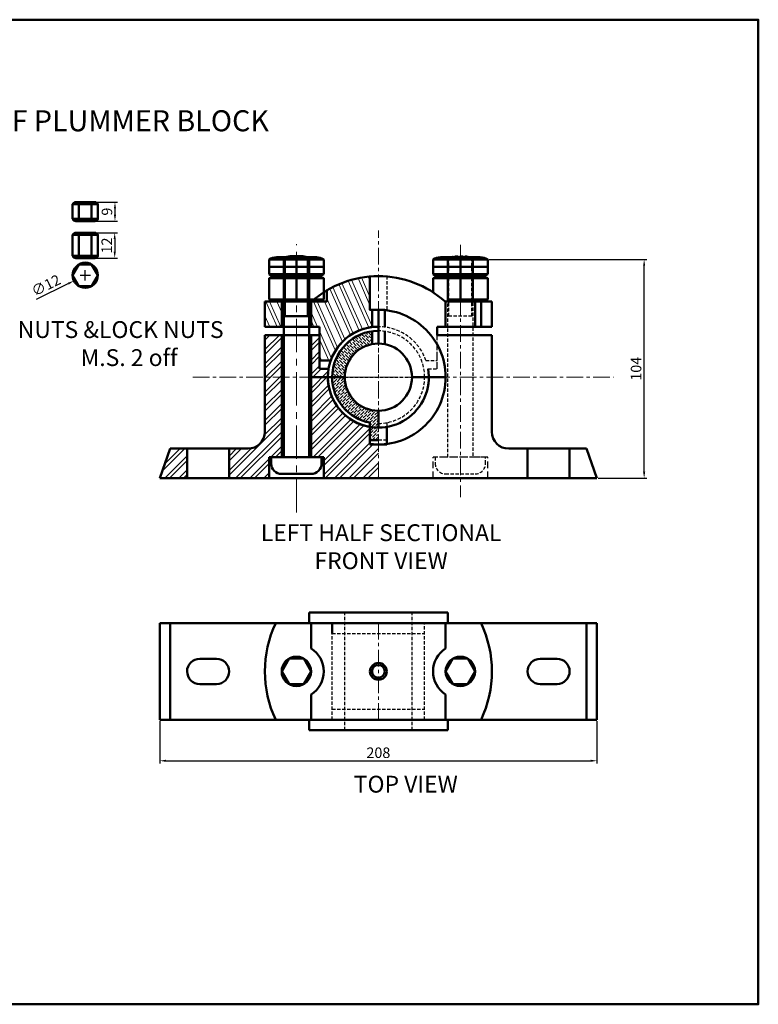
# Model space of a CAD drawing. Units: millimetres. Extents: x 6 to 817, y -61 to 407.
# Tile 3 of 3: x 466 to 817, y -61 to 407. Entities that reach past the tile are written whole.
import ezdxf

# ---------------------------------------------------------------- set-up
doc = ezdxf.new("R2010")
doc.units = ezdxf.units.MM
doc.header["$LTSCALE"] = 0.5
doc.linetypes.add('CENTER', pattern=[50.8, 31.75, -6.35, 6.35, -6.35])
doc.linetypes.add('HIDDEN', pattern=[9.525, 6.35, -3.175])
for name, color, linetype, lineweight in [('M-CNTR', 1, 'CENTER', 18), ('M-DIMS', 2, 'Continuous', 25), ('M-HATC', 8, 'Continuous', 18), ('M-HIDN', 4, 'HIDDEN', 25), ('M-OUTL', 7, 'Continuous', 50), ('M-TEXT', 3, 'Continuous', 25)]:
    doc.layers.add(name, color=color, linetype=linetype, lineweight=lineweight)
doc.styles.get("Standard").update_dxf_attribs({"font": 'arial.ttf'})
doc.dimstyles.new('ISO-25', dxfattribs={"dimtxt": 5, "dimasz": 3, "dimexe": 1.25, "dimexo": 0.625, "dimtad": 1, "dimtxsty": 'Standard', "dimcen": 2.5, "dimadec": 0, "dimazin": 0, "dimtfac": 1, "dimtofl": 0, "dimtmove": 0, "dimatfit": 3, "dimfxl": 1, "dimarcsym": 0})

# ---------------------------------------------------------------- blocks, each defined once
blk = doc.blocks.new('*D46')
at = {"layer": 'Defpoints', "color": 0, "ltscale": 0.5, "transparency": 16777216}
for p in [(500.08, 320.46), (500.08, 311.46), (511.22, 311.46)]:
    blk.add_point(p, dxfattribs=at)
at = {"layer": 'M-DIMS', "color": 0, "lineweight": -2, "ltscale": 0.5, "transparency": 16777216}
for p, q in [((500.7, 320.46), (512.47, 320.46)), ((511.22, 317.46), (511.22, 314.46)), ((500.7, 311.46), (512.47, 311.46))]:
    blk.add_line(p, q, dxfattribs=at)
at = {"layer": 'M-DIMS', "color": 0, "ltscale": 0.5, "transparency": 16777216}
for points in [[(510.72, 317.46), (511.72, 317.46), (511.22, 320.46)], [(510.72, 314.46), (511.72, 314.46), (511.22, 311.46)]]:
    blk.add_solid(points, dxfattribs=at)
at = {"layer": 'M-DIMS', "color": 0, "ltscale": 0.5, "transparency": 16777216, "insert": (508.04, 315.96), "char_height": 5, "attachment_point": 5, "rotation": 90}
blk.add_mtext('9', dxfattribs=at)
blk = doc.blocks.new('*D47')
at = {"layer": 'Defpoints', "color": 0, "ltscale": 0.5, "transparency": 16777216}
for p in [(497.09, 305.87), (497.09, 293.87), (511.09, 293.87)]:
    blk.add_point(p, dxfattribs=at)
at = {"layer": 'M-DIMS', "color": 0, "lineweight": -2, "ltscale": 0.5, "transparency": 16777216}
for p, q in [((497.71, 305.87), (512.34, 305.87)), ((511.09, 302.87), (511.09, 296.87)), ((497.71, 293.87), (512.34, 293.87))]:
    blk.add_line(p, q, dxfattribs=at)
at = {"layer": 'M-DIMS', "color": 0, "ltscale": 0.5, "transparency": 16777216}
for points in [[(510.59, 302.87), (511.59, 302.87), (511.09, 305.87)], [(510.59, 296.87), (511.59, 296.87), (511.09, 293.87)]]:
    blk.add_solid(points, dxfattribs=at)
at = {"layer": 'M-DIMS', "color": 0, "ltscale": 0.5, "transparency": 16777216, "insert": (507.95, 299.87), "char_height": 5, "attachment_point": 5, "rotation": 90}
blk.add_mtext('12', dxfattribs=at)
blk = doc.blocks.new('*D48')
at = {"layer": 'Defpoints', "color": 0, "ltscale": 0.5, "transparency": 16777216}
for p in [(502.46, 288.34), (491.69, 283.05)]:
    blk.add_point(p, dxfattribs=at)
at = {"layer": 'M-DIMS', "color": 0, "lineweight": -2, "ltscale": 0.5, "transparency": 16777216}
for p, q in [((494.58, 285.7), (499.58, 285.7)), ((497.08, 283.2), (497.08, 288.2)), ((473.92, 274.32), (489, 281.73))]:
    blk.add_line(p, q, dxfattribs=at)
at = {"layer": 'M-DIMS', "color": 0, "ltscale": 0.5, "transparency": 16777216}
blk.add_solid([(488.78, 282.18), (489.22, 281.28), (491.69, 283.05)], dxfattribs=at)
at = {"layer": 'M-DIMS', "color": 0, "ltscale": 0.5, "transparency": 16777216, "insert": (478.65, 280.34), "char_height": 5, "attachment_point": 5, "rotation": 26.1724}
blk.add_mtext('∅12', dxfattribs=at)
blk = doc.blocks.new('SLOT-BASE')
for p, q in [((6, 12), (14, 12)), ((0, 6), (0, 6)), ((20, 6), (20, 6)), ((6, 0), (14, 0))]:
    blk.add_line(p, q)
for centre, start, end in [((6, 6), 90, 180), ((14, 6), 0, 90), ((6, 6), 180, 270), ((14, 6), 270, 0)]:
    blk.add_arc(centre, 6, start, end)
blk = doc.blocks.new('BOLT-HEAD')
at = {"ltscale": 0.5}
for p, q in [((0, 4.5), (0, 8)), ((26, 4.5), (26, 8)), ((0, 1), (0, 4.5)), ((0, 4.5), (26, 4.5)), ((26, 1), (26, 4.5))]:
    blk.add_line(p, q, dxfattribs=at)
for points in [[(0, 8), (7, 8), (19, 8), (26, 8)], [(26, 1), (19, 1), (7, 1), (0, 1)]]:
    blk.add_lwpolyline(points, dxfattribs=at)
for centre, radius, start, end in [((3.5, 2.38), 6.63, 58.1092, 121.8908), ((13, -9.5), 18.5, 71.0754, 108.9246), ((22.5, 2.38), 6.62, 58.1092, 121.8908), ((3.5, 6.63), 6.62, 238.1092, 301.8908), ((13, 18.5), 18.5, 251.0754, 288.9246), ((22.5, 6.63), 6.62, 238.1092, 301.8908)]:
    blk.add_arc(centre, radius, start, end, dxfattribs=at)
blk = doc.blocks.new('*D55')
at = {"layer": 'Defpoints', "color": 0, "ltscale": 0.5, "transparency": 16777216}
for p in [(532.52, 74.34), (740.52, 74.34), (740.52, 54.84)]:
    blk.add_point(p, dxfattribs=at)
at = {"layer": 'M-DIMS', "color": 0, "lineweight": -2, "ltscale": 0.5, "transparency": 16777216}
for p, q in [((532.52, 73.71), (532.52, 53.59)), ((740.52, 73.71), (740.52, 53.59)), ((535.52, 54.84), (737.52, 54.84))]:
    blk.add_line(p, q, dxfattribs=at)
at = {"layer": 'M-DIMS', "color": 0, "ltscale": 0.5, "transparency": 16777216}
for points in [[(535.52, 55.34), (535.52, 54.34), (532.52, 54.84)], [(737.52, 55.34), (737.52, 54.34), (740.52, 54.84)]]:
    blk.add_solid(points, dxfattribs=at)
at = {"layer": 'M-DIMS', "color": 0, "ltscale": 0.5, "transparency": 16777216, "insert": (636.52, 58.02), "char_height": 5, "attachment_point": 5}
blk.add_mtext('208', dxfattribs=at)
blk = doc.blocks.new('*D56')
at = {"layer": 'Defpoints', "color": 0, "ltscale": 0.5, "transparency": 16777216}
for p in [(688.52, 293.25), (762.95, 293.25), (740.52, 189.25)]:
    blk.add_point(p, dxfattribs=at)
at = {"layer": 'M-DIMS', "color": 0, "lineweight": -2, "ltscale": 0.5, "transparency": 16777216}
for p, q in [((689.14, 293.25), (764.2, 293.25)), ((762.95, 192.25), (762.95, 290.25)), ((741.14, 189.25), (764.2, 189.25))]:
    blk.add_line(p, q, dxfattribs=at)
at = {"layer": 'M-DIMS', "color": 0, "ltscale": 0.5, "transparency": 16777216}
for points in [[(762.45, 290.25), (763.45, 290.25), (762.95, 293.25)], [(762.45, 192.25), (763.45, 192.25), (762.95, 189.25)]]:
    blk.add_solid(points, dxfattribs=at)
at = {"layer": 'M-DIMS', "color": 0, "ltscale": 0.5, "transparency": 16777216, "insert": (759.77, 241.25), "char_height": 5, "attachment_point": 5, "rotation": 90}
blk.add_mtext('104', dxfattribs=at)

msp = doc.modelspace()

# ---------------------------------------------------------------- hatches: boundary and pattern name
at = {"layer": 'M-HATC', "ltscale": 0.5}
h = msp.add_hatch(dxfattribs=at)
h.set_pattern_fill('ANSI32', color=256, scale=0.5, angle=69)
h.set_pattern_definition([(114, (872.1417, 14.299), (-4.35076, -1.937083), []), (114, (872.9463, 16.3947), (-4.35076, -1.937083), [])])
h.paths.add_polyline_path([(633.519, 269.252), (632.519, 269.252), (632.519, 285.085, 0.113544), (612.019, 278.529), (612.019, 273.252), (604.77, 273.252), (604.519, 273.252), (604.519, 261.252), (608.519, 261.252), (608.519, 257.252), (608.519, 245.252), (613.892, 245.252, -0.2836692), (633.519, 261.064)])
h = msp.add_hatch(dxfattribs=at)
h.set_pattern_fill('ANSI32', color=256, scale=0.5, angle=69)
h.set_pattern_definition([(114, (427.4883, -44.975), (-4.35076, -1.937083), []), (114, (428.293, -42.879), (-4.35076, -1.937083), [])])
h.paths.add_polyline_path([(590.519, 273.252), (582.519, 273.252), (582.519, 261.252), (590.519, 261.252)])
h = msp.add_hatch(dxfattribs=at)
h.set_pattern_fill('ANSI36', color=256, scale=0.3, angle=90)
h.set_pattern_definition([(135, (770.454, -107.801), (-1.8521778, 0.5051394), [2.38125, -0.47625, 0, -0.47625])])
h.paths.add_polyline_path([(633.519, 252.969), (633.519, 259.047, 0.3746932), (614.519, 237.252), (620.519, 237.252, -0.359988)])
h = msp.add_hatch(dxfattribs=at)
h.set_pattern_fill('ANSI32', color=256, scale=0.5)
h.set_pattern_definition([(45, (427.4883, 75.1094), (-3.3676, 3.3676), []), (45, (429.7333, 75.1094), (-3.3676, 3.3676), [])])
h.paths.add_polyline_path([(545.519, 203.252), (537.519, 203.252), (532.519, 189.252), (545.519, 189.252)])
h.paths.add_polyline_path([(590.519, 257.252), (582.519, 257.252), (582.519, 211.252, -0.4142136), (574.519, 203.252), (565.519, 203.252), (565.519, 189.252), (584.519, 189.252), (584.519, 199.252), (590.519, 199.252)])
h.paths.add_polyline_path([(632.519, 213.588, -0.4142136), (612.855, 241.252), (608.519, 241.252), (608.519, 257.252), (604.519, 257.252), (604.519, 199.252), (610.519, 199.252), (610.519, 189.252), (636.519, 189.252), (636.519, 205.252), (632.519, 205.252)])
h = msp.add_hatch(dxfattribs=at)
h.set_pattern_fill('ANSI36', color=256, scale=0.3)
h.set_pattern_definition([(45, (770.454, -69.3824), (0.5051394, 1.8521778), [2.38125, -0.47625, 0, -0.47625])])
h.paths.add_polyline_path([(632.519, 215.619), (632.519, 207.252), (636.519, 207.252), (636.519, 221.252, -0.4142136), (620.519, 237.252), (614.519, 237.252, 0.3616215)])

# ---------------------------------------------------------------- linework, layer by layer
at = {"layer": 'M-CNTR', "ltscale": 0.5}
for p, q in [((636.519, 189.252), (636.519, 306.922)), ((675.519, 300.115), (675.519, 180.205)), ((636.519, 272.727), (636.519, 237.252)), ((548.219, 237.252), (748.451, 237.252)), ((636.519, 201.778), (636.519, 237.252)), ((636.519, 74.338), (636.519, 120.338))]:
    msp.add_line(p, q, dxfattribs=at)
at = {"layer": 'M-CNTR'}
msp.add_line((597.519, 172.977), (597.519, 300.562), dxfattribs=at)
at = {"layer": 'M-HIDN', "ltscale": 0.5}
for p, q in [((669.519, 294.252), (681.519, 294.252)), ((669.519, 199.252), (669.519, 294.252)), ((670.019, 266.252), (670.019, 294.35)), ((681.019, 266.252), (681.019, 294.35)), ((681.519, 294.252), (681.519, 199.252)), ((670.019, 266.252), (669.519, 266.752)), ((681.019, 266.252), (670.019, 266.252)), ((681.019, 266.252), (681.519, 266.752)), ((664.519, 245.252), (664.519, 257.252)), ((659.146, 245.252), (664.519, 245.252)), ((660.183, 241.252), (664.519, 241.252)), ((620.519, 237.252), (652.519, 237.252)), ((620.519, 237.252), (652.519, 237.252)), ((640.519, 215.619), (640.519, 207.252)), ((640.519, 207.252), (636.519, 207.252)), ((669.519, 199.252), (663.519, 199.252)), ((663.519, 199.252), (663.519, 196.252)), ((681.519, 199.252), (669.519, 199.252)), ((687.519, 199.252), (681.519, 199.252)), ((687.519, 196.252), (687.519, 199.252)), ((668.519, 191.252), (682.519, 191.252)), ((620.519, 69.338), (620.519, 125.338)), ((652.519, 69.338), (652.519, 125.338)), ((614.519, 74.338), (614.519, 120.338)), ((658.519, 74.338), (658.519, 120.338)), ((614.519, 115.338), (658.519, 115.338)), ((614.519, 79.338), (658.519, 79.338))]:
    msp.add_line(p, q, dxfattribs=at)
at = {"layer": 'M-HIDN'}
for p, q in [((664.519, 241.252), (664.519, 257.252)), ((662.519, 189.252), (662.519, 199.252)), ((688.519, 199.252), (662.519, 199.252)), ((688.519, 189.252), (688.519, 199.252))]:
    msp.add_line(p, q, dxfattribs=at)
at = {"layer": 'M-HIDN', "ltscale": 0.5}
msp.add_lwpolyline([(640.519, 285.252), (640.519, 269.252), (639.519, 269.252)], dxfattribs=at)
for centre, radius, start, end in [((675.519, 264.868), 29.991, 78.45948, 101.54052), ((636.519, 237.252), 24, 19.47122, 90), ((636.519, 237.252), 22, 0, 90), ((636.519, 237.252), 22, 270, 0), ((636.519, 237.252), 24, 270, 0), ((668.519, 196.252), 5, 180, 270), ((682.519, 196.252), 5, 270, 0)]:
    msp.add_arc(centre, radius, start, end, dxfattribs=at)
at = {"layer": 'M-OUTL', "ltscale": 0.5}
for p, q in [((491.079, 315.964), (491.079, 319.464)), ((492.513, 320.464), (501.657, 320.464)), ((503.079, 315.964), (503.079, 319.464)), ((491.079, 312.464), (491.079, 315.964)), ((503.079, 312.464), (503.079, 315.964)), ((492.513, 311.464), (501.657, 311.464)), ((491.079, 294.873), (491.079, 304.873)), ((491.079, 304.873), (503.079, 304.873)), ((492.513, 305.873), (501.657, 305.873)), ((494.079, 293.873), (494.079, 305.873)), ((500.079, 293.873), (500.079, 305.873)), ((503.079, 294.873), (503.079, 304.873)), ((491.079, 294.873), (503.079, 294.873)), ((492.513, 293.873), (501.657, 293.873)), ((591.519, 294.252), (603.519, 294.252)), ((591.519, 199.252), (591.519, 294.252)), ((591.519, 294.252), (591.519, 289.752)), ((592.019, 266.252), (592.019, 294.35)), ((597.519, 294.252), (597.519, 289.752)), ((603.019, 266.252), (603.019, 294.35)), ((603.519, 294.252), (603.519, 199.252)), ((603.519, 294.252), (603.519, 289.752)), ((669.519, 294.252), (669.519, 289.752)), ((675.519, 294.252), (675.519, 289.752)), ((681.519, 294.252), (681.519, 289.752)), ((591.519, 289.752), (591.519, 285.252)), ((597.519, 289.752), (597.519, 285.252)), ((603.519, 289.752), (603.519, 285.252)), ((669.519, 289.752), (669.519, 285.252)), ((675.519, 289.752), (675.519, 285.252)), ((681.519, 289.752), (681.519, 285.252)), ((584.519, 274.252), (584.519, 284.252)), ((591.519, 285.252), (591.519, 273.252)), ((597.519, 285.252), (597.519, 273.252)), ((603.519, 285.252), (603.519, 273.252)), ((610.519, 274.252), (610.519, 284.252)), ((662.519, 277.601), (662.519, 284.252)), ((669.519, 285.252), (669.519, 273.252)), ((675.519, 285.252), (675.519, 273.252)), ((681.519, 285.252), (681.519, 273.252)), ((688.519, 274.252), (688.519, 284.252)), ((604.77, 273.252), (582.519, 273.252)), ((582.519, 273.252), (582.519, 261.252)), ((590.519, 273.252), (590.519, 261.252)), ((604.519, 273.252), (604.519, 261.252)), ((690.519, 273.252), (668.268, 273.252)), ((668.519, 261.252), (668.519, 273.252)), ((682.519, 261.252), (682.519, 273.252)), ((685.376, 261.252), (685.376, 273.252)), ((690.519, 261.252), (690.519, 273.252)), ((690.519, 261.252), (690.519, 273.252)), ((633.519, 261.064), (633.519, 269.252)), ((636.519, 261.252), (636.519, 269.252)), ((636.519, 269.252), (639.519, 269.252)), ((639.519, 269.252), (639.519, 261.252)), ((592.019, 266.252), (591.519, 266.752)), ((603.019, 266.252), (592.019, 266.252)), ((603.019, 266.252), (603.519, 266.752)), ((582.519, 261.252), (608.519, 261.252)), ((608.519, 261.252), (608.519, 257.252)), ((633.519, 259.047), (633.519, 252.969)), ((636.519, 259.252), (636.519, 261.252)), ((636.519, 261.252), (636.519, 253.252)), ((639.519, 259.047), (639.519, 252.969)), ((664.519, 257.252), (664.519, 261.252)), ((664.519, 261.252), (690.519, 261.252)), ((608.519, 257.252), (608.519, 245.252)), ((608.519, 245.252), (613.892, 245.252)), ((608.519, 241.252), (612.855, 241.252)), ((604.519, 237.252), (620.519, 237.252)), ((604.519, 237.252), (620.519, 237.252)), ((652.519, 237.252), (668.519, 237.252)), ((652.519, 237.252), (668.519, 237.252)), ((636.519, 213.252), (636.519, 221.252)), ((632.519, 215.619), (632.519, 207.252)), ((632.519, 213.588), (632.519, 205.252)), ((640.519, 205.252), (640.519, 213.588)), ((636.519, 207.252), (632.519, 207.252)), ((632.519, 205.252), (640.519, 205.252)), ((591.519, 199.252), (585.519, 199.252)), ((585.519, 199.252), (585.519, 196.252)), ((603.519, 199.252), (591.519, 199.252)), ((609.519, 199.252), (603.519, 199.252)), ((609.519, 196.252), (609.519, 199.252)), ((590.519, 191.252), (604.519, 191.252)), ((603.519, 120.338), (603.521, 125.338)), ((603.521, 125.338), (669.519, 125.338)), ((669.519, 125.338), (669.519, 120.338)), ((604.519, 108.292), (604.519, 120.338)), ((614.519, 120.338), (614.519, 115.338)), ((668.519, 108.292), (668.519, 120.338)), ((604.519, 86.383), (604.519, 74.338)), ((668.519, 86.383), (668.519, 74.338)), ((603.519, 74.338), (603.521, 69.338)), ((669.519, 69.338), (669.519, 74.338)), ((603.521, 69.338), (669.519, 69.338))]:
    msp.add_line(p, q, dxfattribs=at)
at = {"layer": 'M-OUTL'}
for p, q in [((582.519, 257.252), (608.519, 257.252)), ((582.519, 211.252), (582.519, 257.252)), ((590.519, 199.252), (590.519, 257.252)), ((604.519, 199.252), (604.519, 257.252)), ((608.519, 241.252), (608.519, 257.252)), ((664.519, 257.252), (690.519, 257.252)), ((690.519, 211.252), (690.519, 257.252)), ((532.519, 189.252), (537.519, 203.252)), ((574.519, 203.252), (537.519, 203.252)), ((545.519, 203.252), (545.519, 189.252)), ((565.519, 203.252), (565.519, 189.252)), ((735.519, 203.252), (698.519, 203.252)), ((707.519, 203.252), (707.519, 189.252)), ((727.519, 203.252), (727.519, 189.252)), ((740.519, 189.252), (735.519, 203.252)), ((584.519, 189.252), (584.519, 199.252)), ((610.519, 199.252), (584.519, 199.252)), ((610.519, 189.252), (610.519, 199.252)), ((610.519, 189.252), (610.519, 199.252)), ((532.519, 189.252), (740.519, 189.252)), ((532.519, 120.338), (740.519, 120.338)), ((532.519, 74.338), (532.519, 120.338)), ((537.519, 120.338), (537.519, 74.338)), ((735.519, 120.338), (735.519, 74.338)), ((740.519, 120.338), (740.519, 74.338)), ((740.519, 74.338), (532.519, 74.338))]:
    msp.add_line(p, q, dxfattribs=at)
at = {"layer": 'M-OUTL', "ltscale": 0.5}
for points in [[(6.354, 407.228), (817.271, 407.228), (817.271, -60.955), (6.354, -60.955)], [(503.079, 285.697), (500.079, 290.894), (494.079, 290.894), (491.079, 285.697), (494.079, 280.501), (500.079, 280.501)], [(604.519, 97.338), (601.019, 103.4), (594.019, 103.4), (590.519, 97.338), (594.019, 91.275), (601.019, 91.275)], [(682.519, 97.338), (679.019, 103.4), (672.019, 103.4), (668.519, 97.338), (672.019, 91.275), (679.019, 91.275)]]:
    msp.add_lwpolyline(points, close=True, dxfattribs=at)
for points in [[(503.079, 319.464, 0.6679377), (500.079, 319.464, 0.3333333), (494.079, 319.464, 0.6675542), (491.079, 319.464)], [(491.079, 312.464, 0.6675542), (494.079, 312.464, 0.3333333), (500.079, 312.464, 0.6679377), (503.079, 312.464)]]:
    msp.add_lwpolyline(points, format="xyb", close=True, dxfattribs=at)
for points in [[(494.079, 311.464), (494.079, 315.964), (494.079, 320.464)], [(500.079, 311.464), (500.079, 315.964), (500.079, 320.464)], [(588.019, 294.252), (591.519, 294.252), (603.519, 294.252), (607.019, 294.252)], [(666.019, 294.252), (669.519, 294.252), (681.519, 294.252), (685.019, 294.252)], [(584.519, 284.252), (591.519, 284.252), (603.519, 284.252), (610.519, 284.252)], [(588.019, 285.252), (591.519, 285.252), (603.519, 285.252), (607.019, 285.252)], [(607.019, 285.252), (603.519, 285.252), (591.519, 285.252), (588.019, 285.252)], [(632.519, 285.252), (632.519, 269.252), (636.519, 269.252)], [(662.519, 284.252), (669.519, 284.252), (681.519, 284.252), (688.519, 284.252)], [(666.019, 285.252), (669.519, 285.252), (681.519, 285.252), (685.019, 285.252)], [(685.019, 285.252), (681.519, 285.252), (669.519, 285.252), (666.019, 285.252)], [(604.77, 273.252), (612.019, 273.252), (612.019, 278.529)], [(610.519, 274.252), (603.519, 274.252), (591.519, 274.252), (584.519, 274.252)], [(607.019, 273.252), (603.519, 273.252), (591.519, 273.252), (588.019, 273.252)], [(685.019, 273.252), (681.519, 273.252), (669.519, 273.252), (668.268, 273.252)], [(688.519, 274.252), (681.519, 274.252), (669.519, 274.252)]]:
    msp.add_lwpolyline(points, dxfattribs=at)
for centre, radius in [((497.079, 285.697), 6), ((636.519, 97.338), 3)]:
    msp.add_circle(centre, radius, dxfattribs=at)
at = {"layer": 'M-OUTL'}
for centre, radius in [((597.519, 97.338), 7), ((675.519, 97.338), 7), ((636.519, 97.338), 4)]:
    msp.add_circle(centre, radius, dxfattribs=at)
at = {"layer": 'M-OUTL', "ltscale": 0.5}
for centre, radius, start, end in [((492.579, 304.25), 1.624, 22.54949, 157.45051), ((497.079, 300.873), 5, 53.1301, 126.8699), ((501.579, 304.251), 1.624, 22.51909, 157.48091), ((492.579, 295.496), 1.624, 202.54949, 337.45051), ((497.079, 298.873), 5, 233.1301, 306.8699), ((501.579, 295.495), 1.624, 202.51909, 337.48091), ((597.519, 264.868), 29.991, 78.45948, 101.54052), ((588.019, 278.627), 6.625, 58.10921, 121.89079), ((597.519, 266.752), 18.5, 71.07536, 108.92464), ((607.019, 278.627), 6.625, 58.10921, 121.89079), ((636.519, 237.252), 48, 90, 131.40962), ((636.519, 237.252), 48, 48.59038, 90), ((666.019, 278.627), 6.625, 58.10921, 121.89079), ((675.519, 266.752), 18.5, 71.07536, 108.92464), ((685.019, 278.627), 6.625, 58.10921, 121.89079), ((588.019, 279.877), 6.625, 238.10921, 301.89079), ((597.519, 291.752), 18.5, 251.07535, 288.92465), ((607.019, 279.877), 6.625, 238.10921, 301.89079), ((675.519, 291.752), 18.5, 251.07535, 288.92465), ((685.019, 279.877), 6.625, 238.10921, 301.89079), ((636.519, 237.252), 32, 0, 95.37938), ((636.519, 237.252), 24, 90, 180), ((636.519, 237.252), 24, 90, 160.52878), ((636.519, 237.252), 22, 90, 180), ((636.519, 237.252), 16, 0, 180), ((636.519, 237.252), 24, 180, 260.40593), ((636.519, 237.252), 22, 180, 259.52432), ((636.519, 237.252), 16, 180, 0), ((636.519, 237.252), 32, 262.81924, 0), ((590.519, 196.252), 5, 180, 270), ((604.519, 196.252), 5, 270, 0), ((597.519, 97.338), 13, 302.57897, 57.42103), ((675.519, 97.338), 13, 122.57897, 237.42103), ((675.519, 97.338), 13, 122.57897, 237.42103)]:
    msp.add_arc(centre, radius, start, end, dxfattribs=at)
at = {"layer": 'M-OUTL'}
for centre, radius, start, end in [((636.519, 237.252), 24, 170.40593, 9.59407), ((574.519, 211.252), 8, 270, 0), ((698.519, 211.252), 8, 180, 270), ((636.519, 97.338), 54, 154.79071, 205.20929), ((636.519, 97.338), 54, 334.79071, 25.20929)]:
    msp.add_arc(centre, radius, start, end, dxfattribs=at)

# ---------------------------------------------------------------- block references
for name, p in [('BOLT-HEAD', (584.519, 285.252)), ('BOLT-HEAD', (662.519, 285.252)), ('SLOT-BASE', (707.519, 91.338))]:
    msp.add_blockref(name, p, dxfattribs=at)
at = {"layer": 'M-OUTL', "rotation": 180}
msp.add_blockref('SLOT-BASE', (565.519, 103.337), dxfattribs=at)

# ---------------------------------------------------------------- texts
at = {"layer": 'M-TEXT', "ltscale": 0.5, "attachment_point": 1}
for s, width, insert, char_height in [('ASSEMBLY DRAWING OF PLUMMER BLOCK', 345.85464, (316.953, 364.17), 10), ('\\pxqc;NUTS &LOCK NUTS\\P\\pi-3,l4,t4;M.S.^I2 off', 106.37362, (460.728, 263.878), 8), ('\\pxqc;LEFT HALF SECTIONAL FRONT VIEW', 148.01432, (563.817, 167.295), 8), ('\\pxqc;TOP VIEW', 106.37362, (596.369, 47.714), 8)]:
    msp.add_mtext_dynamic_manual_height_columns(s, width=width, gutter_width=12.5, heights=[0], dxfattribs=dict(at, insert=insert, char_height=char_height))

# ---------------------------------------------------------------- dimensions: what is measured, and where the dimension line sits
at = {"layer": 'M-DIMS', "ltscale": 0.5}
for base, p1, p2, override, picture, middle in [((511.222, 311.464), (500.079, 320.464), (500.079, 311.464), {"dimclrd": 0, "dimclre": 0, "dimclrt": 0}, '*D46', (508.044, 315.964)), ((511.088, 293.873), (497.085, 305.873), (497.085, 293.873), {"dimclrd": 0, "dimclre": 0, "dimclrt": 0}, '*D47', (507.953, 299.873)), ((762.951, 293.252), (740.519, 189.252), (688.519, 293.252), {"dimdec": 0, "dimlfac": 1, "dimrnd": 0, "dimzin": 0, "dimdsep": 46, "dimlunit": 2}, '*D56', (759.773, 241.252))]:
    dim = msp.add_linear_dim(base=base, p1=p1, p2=p2, angle=90, dimstyle='ISO-25', override=override, dxfattribs=at)
    dim.commit()
    dim.dimension.update_dxf_attribs({"geometry": picture, "text_midpoint": middle})
dim = msp.add_diameter_dim_2p(p1=(502.464, 288.344), p2=(491.694, 283.051), dimstyle='ISO-25', override={"dimclrd": 0, "dimclre": 0, "dimclrt": 0}, dxfattribs=at)
dim.commit()
dim.dimension.update_dxf_attribs({"geometry": '*D48', "text_midpoint": (478.653, 280.338)})
dim = msp.add_linear_dim(base=(740.519, 54.838), p1=(532.519, 74.338), p2=(740.519, 74.338), dimstyle='ISO-25', override={"dimdec": 0, "dimlfac": 1, "dimrnd": 0, "dimzin": 0, "dimdsep": 46, "dimlunit": 2}, dxfattribs=at)
dim.commit()
dim.dimension.update_dxf_attribs({"geometry": '*D55', "text_midpoint": (636.519, 58.015)})

doc.saveas('drawing.dxf')
